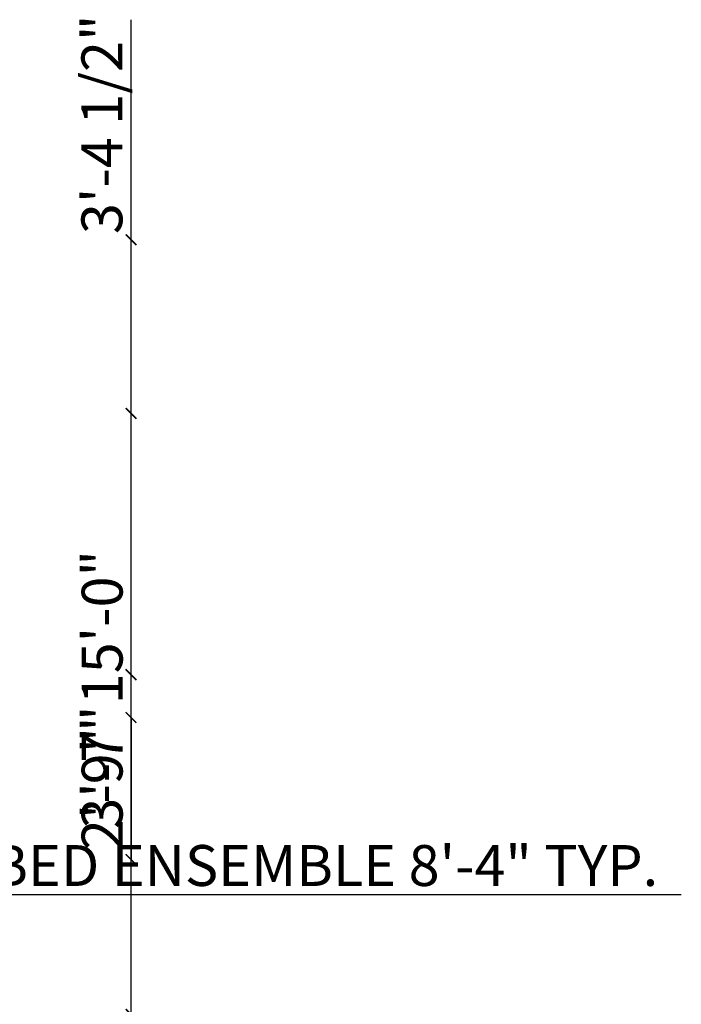
# Model space of a CAD drawing. Units: inches. Extents: x 1704 to 2334, y 1856 to 2559.
# Tile 10 of 10: x 2180 to 2334, y 2321 to 2550. Entities that reach past the tile are written whole.
import ezdxf

# ---------------------------------------------------------------- set-up
doc = ezdxf.new("R2010")
doc.units = ezdxf.units.IN
doc.layers.add('A-ANNO-DIMS', color=2, linetype='Continuous', lineweight=18)
doc.styles.get("Standard").update_dxf_attribs({"font": 'arial.ttf'})
doc.dimstyles.new('ISO-25', dxfattribs={"dimtxt": 9.5, "dimasz": 2.5, "dimexe": 1.25, "dimexo": 0.625, "dimtad": 1, "dimdec": 0, "dimlunit": 4, "dimtxsty": 'Standard', "dimblk": 'ARCHTICK', "dimcen": 2.5, "dimse1": 1, "dimse2": 1, "dimclrd": 3, "dimadec": 0, "dimazin": 0, "dimtfac": 1, "dimtdec": 0, "dimtmove": 0, "dimatfit": 3, "dimfxl": 1, "dimarcsym": 0})

# ---------------------------------------------------------------- blocks, each defined once
blk = doc.blocks.new('_ArchTick')
at = {"color": 0, "linetype": 'ByBlock', "const_width": 0.15}
blk.add_lwpolyline([(-0.5, -0.5), (0.5, 0.5)], dxfattribs=at)
blk = doc.blocks.new('*D24')
at = {"layer": 'A-ANNO-DIMS', "color": 3, "lineweight": -2, "transparency": 16777216}
for p, q in [((2066.27, 2346.88), (2166.04, 2346.88)), ((2166.04, 2346.88), (2334.22, 2346.88))]:
    blk.add_line(p, q, dxfattribs=at)
at = {"layer": 'Defpoints', "color": 0, "transparency": 16777216}
for p in [(2066.27, 2361.85), (2166.04, 2361.85), (2166.04, 2346.88)]:
    blk.add_point(p, dxfattribs=at)
at = {"layer": 'A-ANNO-DIMS', "color": 3, "lineweight": -2, "transparency": 16777216, "xscale": 2.5, "yscale": 2.5, "zscale": 2.5, "rotation": 180}
blk.add_blockref('_ArchTick', (2066.27, 2346.88), dxfattribs=at)
at = {"layer": 'A-ANNO-DIMS', "color": 3, "lineweight": -2, "transparency": 16777216, "xscale": 2.5, "yscale": 2.5, "zscale": 2.5}
blk.add_blockref('_ArchTick', (2166.04, 2346.88), dxfattribs=at)
at = {"layer": 'A-ANNO-DIMS', "color": 0, "transparency": 16777216, "insert": (2251.38, 2352.42), "char_height": 9.5, "attachment_point": 5}
blk.add_mtext('BED ENSEMBLE 8\'-4" TYP.', dxfattribs=at)
blk = doc.blocks.new('*D36')
at = {"layer": 'A-ANNO-DIMS', "color": 3, "lineweight": -2, "transparency": 16777216}
blk.add_line((2206.36, 2319.04), (2206.36, 2499.04), dxfattribs=at)
at = {"layer": 'Defpoints', "color": 0, "transparency": 16777216}
for p in [(2166.01, 2499.04), (2206.36, 2499.04), (2166.01, 2319.04)]:
    blk.add_point(p, dxfattribs=at)
at = {"layer": 'A-ANNO-DIMS', "color": 3, "lineweight": -2, "transparency": 16777216, "xscale": 2.5, "yscale": 2.5, "zscale": 2.5}
for p, rotation in [((2206.36, 2499.04), 90), ((2206.36, 2319.04), 270)]:
    blk.add_blockref('_ArchTick', p, dxfattribs=dict(at, rotation=rotation))
at = {"layer": 'A-ANNO-DIMS', "color": 0, "transparency": 16777216, "insert": (2200.88, 2409.04), "char_height": 9.5, "attachment_point": 5, "rotation": 90}
blk.add_mtext('15\'-0"', dxfattribs=at)
blk = doc.blocks.new('*D69')
at = {"layer": 'A-ANNO-DIMS', "color": 3, "lineweight": -2, "transparency": 16777216}
blk.add_line((2206.36, 2355.04), (2206.36, 2398.02), dxfattribs=at)
at = {"layer": 'Defpoints', "color": 0, "transparency": 16777216}
for p in [(1927.01, 2398.02), (2206.36, 2398.02), (1927.01, 2355.04)]:
    blk.add_point(p, dxfattribs=at)
at = {"layer": 'A-ANNO-DIMS', "color": 3, "lineweight": -2, "transparency": 16777216, "xscale": 2.5, "yscale": 2.5, "zscale": 2.5}
for p, rotation in [((2206.36, 2398.02), 90), ((2206.36, 2355.04), 270)]:
    blk.add_blockref('_ArchTick', p, dxfattribs=dict(at, rotation=rotation))
at = {"layer": 'A-ANNO-DIMS', "color": 0, "transparency": 16777216, "insert": (2200.88, 2376.53), "char_height": 9.5, "attachment_point": 5, "rotation": 90}
blk.add_mtext('3\'-7"', dxfattribs=at)
blk = doc.blocks.new('*D83')
at = {"layer": 'A-ANNO-DIMS', "color": 3, "lineweight": -2, "transparency": 16777216}
for p, q in [((2206.36, 2499.04), (2206.36, 2550.17)), ((2206.36, 2458.69), (2206.36, 2499.04))]:
    blk.add_line(p, q, dxfattribs=at)
at = {"layer": 'Defpoints', "color": 0, "transparency": 16777216}
for p in [(2166.01, 2499.04), (2206.36, 2499.04), (2166.04, 2458.69)]:
    blk.add_point(p, dxfattribs=at)
at = {"layer": 'A-ANNO-DIMS', "color": 3, "lineweight": -2, "transparency": 16777216, "xscale": 2.5, "yscale": 2.5, "zscale": 2.5}
for p, rotation in [((2206.36, 2499.04), 90), ((2206.36, 2458.69), 270)]:
    blk.add_blockref('_ArchTick', p, dxfattribs=dict(at, rotation=rotation))
at = {"layer": 'A-ANNO-DIMS', "color": 0, "transparency": 16777216, "insert": (2200.82, 2525.86), "char_height": 9.5, "attachment_point": 5, "rotation": 90}
blk.add_mtext('3\'-4 1/2"', dxfattribs=at)
blk = doc.blocks.new('*D84')
at = {"layer": 'A-ANNO-DIMS', "color": 3, "lineweight": -2, "transparency": 16777216}
blk.add_line((2206.36, 2388.04), (2206.36, 2355.04), dxfattribs=at)
at = {"layer": 'Defpoints', "color": 0, "transparency": 16777216}
for p in [(1958.54, 2388.04), (1969.04, 2355.04), (2206.36, 2355.04)]:
    blk.add_point(p, dxfattribs=at)
at = {"layer": 'A-ANNO-DIMS', "color": 3, "lineweight": -2, "transparency": 16777216, "xscale": 2.5, "yscale": 2.5, "zscale": 2.5}
for p, rotation in [((2206.36, 2388.04), 90), ((2206.36, 2355.04), 270)]:
    blk.add_blockref('_ArchTick', p, dxfattribs=dict(at, rotation=rotation))
at = {"layer": 'A-ANNO-DIMS', "color": 0, "transparency": 16777216, "insert": (2200.88, 2371.54), "char_height": 9.5, "attachment_point": 5, "rotation": 90}
blk.add_mtext('2\'-9"', dxfattribs=at)

msp = doc.modelspace()

# ---------------------------------------------------------------- dimensions: what is measured, and where the dimension line sits
at = {"layer": 'A-ANNO-DIMS'}
for base, p1, p2, picture, middle in [((2206.3597, 2499.0395), (2166.0449, 2458.6866), (2166.0097, 2499.0395), '*D83', (2200.8195, 2525.8562)), ((2206.36, 2499.04), (2166.01, 2319.04), (2166.01, 2499.04), '*D36', (2200.88, 2409.04)), ((2206.36, 2398.02), (1927.01, 2355.04), (1927.01, 2398.02), '*D69', (2200.88, 2376.53)), ((2206.36, 2355.04), (1958.54, 2388.04), (1969.04, 2355.04), '*D84', (2200.88, 2371.54))]:
    dim = msp.add_linear_dim(base=base, p1=p1, p2=p2, angle=90, dimstyle='ISO-25', override={"dimdec": 1, "dimlfac": 1, "dimrnd": 0, "dimzin": 1, "dimdsep": 46, "dimlunit": 4, "dimfrac": 2}, dxfattribs=at)
    dim.commit()
    dim.dimension.update_dxf_attribs({"geometry": picture, "text_midpoint": middle})
dim = msp.add_linear_dim(base=(2166.04, 2346.88), p1=(2066.27, 2361.85), p2=(2166.04, 2361.85), text='BED ENSEMBLE <> TYP.', dimstyle='ISO-25', override={"dimdec": 1, "dimlfac": 1, "dimrnd": 0, "dimzin": 1, "dimdsep": 46, "dimlunit": 4, "dimfrac": 2}, dxfattribs=at)
dim.commit()
dim.dimension.update_dxf_attribs({"geometry": '*D24', "text_midpoint": (2251.38, 2352.42)})

doc.saveas('drawing.dxf')
